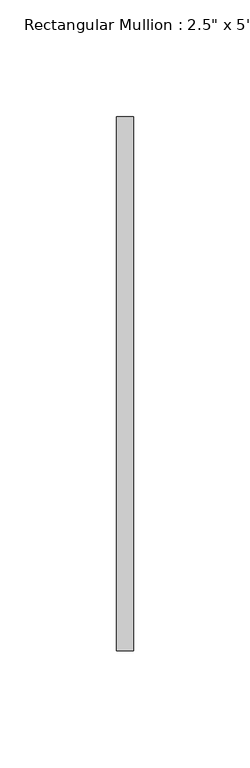
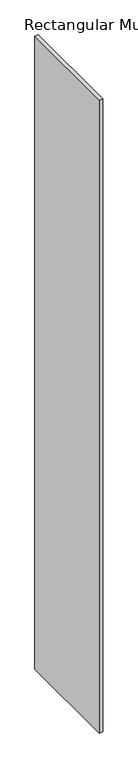
"""IFC4 building model written with IfcOpenShell, lengths in millimetres: member geometry."""

from ifc_helpers import new_model, si_unit, frame, origin, place, context, project, spatial, polyline, outline, extrude, source, transform, mapped, element, save


def member_15c0e2f7(model_context):
    return source(origin(), model_context, "Body", "SweptSolid", [
        extrude(outline(polyline([(0.0, 114.3), (0.0, -114.3), (-7.239, -114.3), (-7.239, 114.3), (0.0, 114.3)])), frame((0.0, 0.0, -1371.6), z_axis=(0.0, 0.0, 1.0), x_axis=(1.0, 0.0, 0.0)), (0.0, 0.0, 1.0), 1371.6),
    ])


if __name__ == "__main__":
    model = new_model("IFC4")
    model_context = context("Model", 3, world=origin())
    ifc_project = project(units=[si_unit("LENGTHUNIT", "METRE", prefix="MILLI")], contexts=[model_context])
    site = spatial("IfcSite", under=ifc_project)
    building = spatial("IfcBuilding", under=site)
    placement = place(None, origin())
    member_shape = member_15c0e2f7(model_context)
    element("IfcMember", 1, ObjectType="Rectangular Mullion : 2.5\" x 5\" rectangular", at=placement, inside=building, context=model_context, shape_type="MappedRepresentation", body=[
        mapped(member_shape, transform((0.0, 0.0, 0.0), x_axis=(1.0, 0.0, 0.0), y_axis=(0.0, 1.0, 0.0), z_axis=(0.0, 0.0, 1.0))),
    ])
    save(model, "model.ifc")

# Revit data of these elements
# Type "Rectangular Mullion : 2.5\" x 5\" rectangular"
#   built-in parameter 1007304 = 0.75 (stored number, unit not read)
#   built-in parameter 1007301 = 0.011875 (stored number, unit not read)
#   built-in parameter 1007300 = 0.011875 (stored number, unit not read)
# Element 1 (IfcMember, "Rectangular Mullion : 2.5\" x 5\" rectangular")
#   Materials on its faces: "WINDOW GLASS MATERIAL"
# Materials
#   "WINDOW GLASS MATERIAL": class "Generic", colour RGB 120 120 120, transparency 0, Cost = 0
